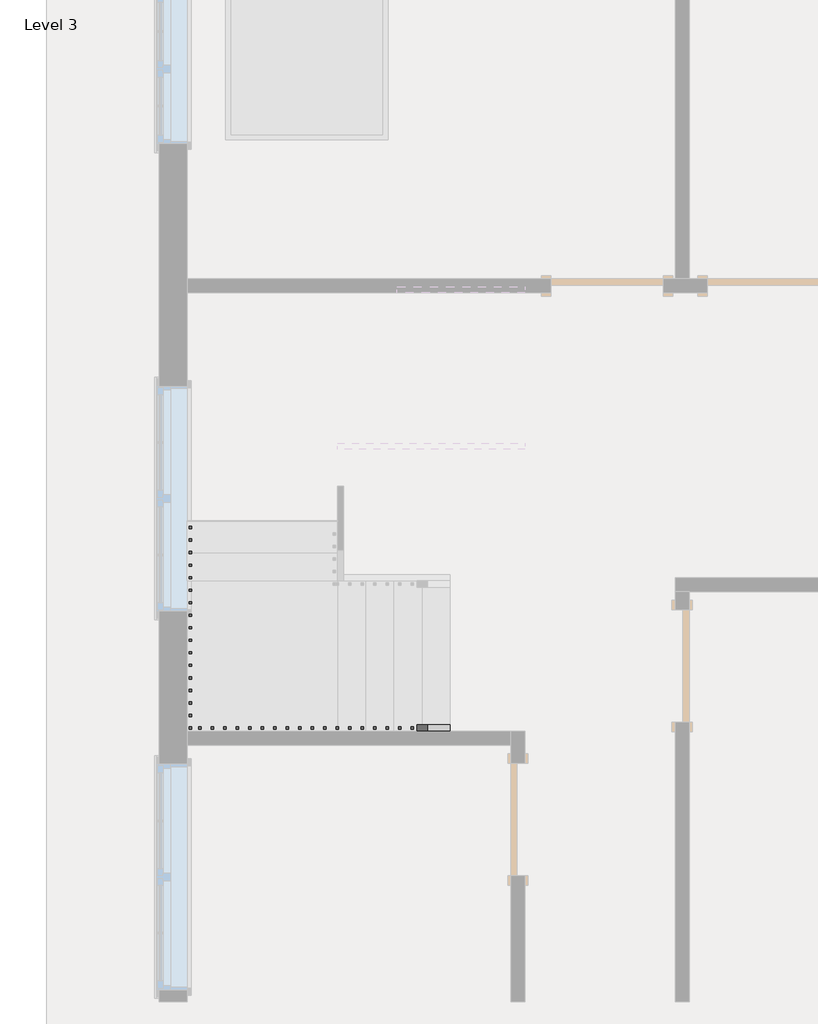
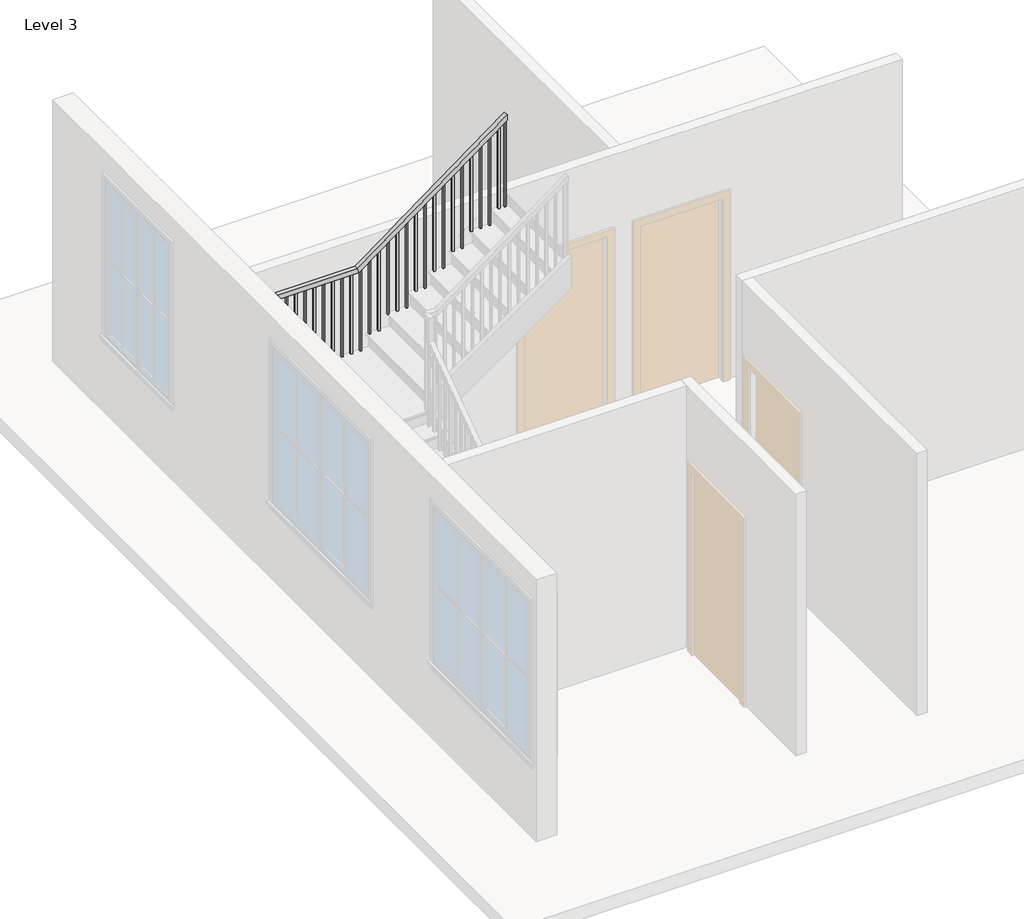
# One storey, part 2 of 3: 1 railing.
"""IFC4 building model written with IfcOpenShell, lengths in millimetres."""

from ifc_helpers import new_model, si_unit, frame, origin, place, context, project, spatial, polyline, outline, extrude, faceted_brep, element, save

model = new_model("IFC4")

# Units and contexts
model_context = context("Model", 3, world=origin())
ifc_project = project(units=[si_unit("LENGTHUNIT", "METRE", prefix="MILLI")], contexts=[model_context])

# Site, building, storey
site = spatial("IfcSite", under=ifc_project)
building = spatial("IfcBuilding", under=site)
storey = spatial("IfcBuildingStorey", under=building, Name="Level 3", Elevation=6248.4)

# Railing
placement = place(None, origin())
element("IfcRailing", 1, ObjectType="Handrail - Rectangular", at=placement, inside=storey, context=model_context, shape_type="SolidModel", body=[
    faceted_brep([(-2683.1105391, -2741.0373761, 7323.2210526), (-2683.1105391, -2741.0373761, 7261.1605986), (-2683.1105391, -2690.2373761, 7261.1605986), (-2683.1105391, -2690.2373761, 7323.2210526), (-3698.24463, -2741.0373761, 8035.5958533), (-3714.290777, -2741.0373761, 7984.7958533), (-3714.290777, -2690.2373761, 7984.7958533), (-3698.24463, -2690.2373761, 8035.5958533), (-4816.7105391, -2741.0373761, 8035.5958533), (-4816.7105391, -2741.0373761, 7984.7958533), (-4765.9105391, -2690.2373761, 7984.7958533), (-4765.9105391, -2690.2373761, 8035.5958533), (-4816.7105391, -1646.8618205, 8035.5958533), (-4816.7105391, -1630.5188912, 7984.7958533), (-4765.9105391, -1630.5188912, 7984.7958533), (-4765.9105391, -1646.8618205, 8035.5958533), (-4816.7105391, -308.3947094, 8996.2181818), (-4816.7105391, -292.0517801, 8945.4181818), (-4765.9105391, -292.0517801, 8945.4181818), (-4765.9105391, -308.3947094, 8996.2181818), (-4816.7105391, 814.9626239, 8996.2181818), (-4816.7105391, 814.9626239, 8945.4181818), (-4765.9105391, 764.1626239, 8945.4181818), (-4765.9105391, 764.1626239, 8996.2181818), (-3721.871578, 814.9626239, 8996.2181818), (-3705.1770744, 814.9626239, 8945.4181818), (-3705.1770744, 764.1626239, 8945.4181818), (-3721.871578, 764.1626239, 8996.2181818), (-2073.5105391, 814.9626239, 10210.8), (-2073.5105391, 764.1626239, 10210.8), (-2073.5105391, 764.1626239, 10147.6987868), (-2073.5105391, 814.9626239, 10147.6987868)], [[[0, 1, 2, 3]], [[1, 0, 4, 5]], [[2, 1, 5, 6]], [[3, 2, 6, 7]], [[0, 3, 7, 4]], [[5, 4, 8, 9]], [[6, 5, 9, 10]], [[7, 6, 10, 11]], [[4, 7, 11, 8]], [[9, 8, 12, 13]], [[10, 9, 13, 14]], [[11, 10, 14, 15]], [[8, 11, 15, 12]], [[13, 12, 16, 17]], [[14, 13, 17, 18]], [[15, 14, 18, 19]], [[12, 15, 19, 16]], [[17, 16, 20, 21]], [[18, 17, 21, 22]], [[19, 18, 22, 23]], [[16, 19, 23, 20]], [[21, 20, 24, 25]], [[22, 21, 25, 26]], [[23, 22, 26, 27]], [[20, 23, 27, 24]], [[28, 29, 30, 31]], [[25, 24, 28, 31]], [[26, 25, 31, 30]], [[27, 26, 30, 29]], [[24, 27, 29, 28]]]),
    extrude(outline(polyline([(10084.5329974, -2159.2355391), (9135.9789474, -2159.2355391), (9135.9789474, -2140.1855391), (10098.5698395, -2140.1855391), (10084.5329974, -2159.2355391)])), frame((0.0, 780.0376239, 0.0), z_axis=(0.0, 1.0, 0.0), x_axis=(0.0, 0.0, 1.0)), (0.0, 0.0, 1.0), 19.05),
    extrude(outline(polyline([(10009.6698395, -2260.8355391), (8975.5578947, -2260.8355391), (8975.5578947, -2241.7855391), (10023.7066816, -2241.7855391), (10009.6698395, -2260.8355391)])), frame((0.0, 780.0376239, 0.0), z_axis=(0.0, 1.0, 0.0), x_axis=(0.0, 0.0, 1.0)), (0.0, 0.0, 1.0), 19.05),
    extrude(outline(polyline([(9934.8066816, -2362.4355391), (8975.5578947, -2362.4355391), (8975.5578947, -2343.3855391), (9948.8435237, -2343.3855391), (9934.8066816, -2362.4355391)])), frame((0.0, 780.0376239, 0.0), z_axis=(0.0, 1.0, 0.0), x_axis=(0.0, 0.0, 1.0)), (0.0, 0.0, 1.0), 19.05),
    extrude(outline(polyline([(9859.9435237, -2464.0355391), (8975.5578947, -2464.0355391), (8975.5578947, -2444.9855391), (9873.9803658, -2444.9855391), (9859.9435237, -2464.0355391)])), frame((0.0, 780.0376239, 0.0), z_axis=(0.0, 1.0, 0.0), x_axis=(0.0, 0.0, 1.0)), (0.0, 0.0, 1.0), 19.05),
    extrude(outline(polyline([(9785.0803658, -2565.6355391), (8815.1368421, -2565.6355391), (8815.1368421, -2546.5855391), (9799.1172079, -2546.5855391), (9785.0803658, -2565.6355391)])), frame((0.0, 780.0376239, 0.0), z_axis=(0.0, 1.0, 0.0), x_axis=(0.0, 0.0, 1.0)), (0.0, 0.0, 1.0), 19.05),
    extrude(outline(polyline([(9710.2172079, -2667.2355391), (8815.1368421, -2667.2355391), (8815.1368421, -2648.1855391), (9724.25405, -2648.1855391), (9710.2172079, -2667.2355391)])), frame((0.0, 780.0376239, 0.0), z_axis=(0.0, 1.0, 0.0), x_axis=(0.0, 0.0, 1.0)), (0.0, 0.0, 1.0), 19.05),
    extrude(outline(polyline([(9635.35405, -2768.8355391), (8654.7157895, -2768.8355391), (8654.7157895, -2749.7855391), (9649.3908921, -2749.7855391), (9635.35405, -2768.8355391)])), frame((0.0, 780.0376239, 0.0), z_axis=(0.0, 1.0, 0.0), x_axis=(0.0, 0.0, 1.0)), (0.0, 0.0, 1.0), 19.05),
    extrude(outline(polyline([(9560.4908921, -2870.4355391), (8654.7157895, -2870.4355391), (8654.7157895, -2851.3855391), (9574.5277342, -2851.3855391), (9560.4908921, -2870.4355391)])), frame((0.0, 780.0376239, 0.0), z_axis=(0.0, 1.0, 0.0), x_axis=(0.0, 0.0, 1.0)), (0.0, 0.0, 1.0), 19.05),
    extrude(outline(polyline([(9485.6277342, -2972.0355391), (8494.2947368, -2972.0355391), (8494.2947368, -2952.9855391), (9499.6645763, -2952.9855391), (9485.6277342, -2972.0355391)])), frame((0.0, 780.0376239, 0.0), z_axis=(0.0, 1.0, 0.0), x_axis=(0.0, 0.0, 1.0)), (0.0, 0.0, 1.0), 19.05),
    extrude(outline(polyline([(9410.7645763, -3073.6355391), (8494.2947368, -3073.6355391), (8494.2947368, -3054.5855391), (9424.8014184, -3054.5855391), (9410.7645763, -3073.6355391)])), frame((0.0, 780.0376239, 0.0), z_axis=(0.0, 1.0, 0.0), x_axis=(0.0, 0.0, 1.0)), (0.0, 0.0, 1.0), 19.05),
    extrude(outline(polyline([(9335.9014184, -3175.2355391), (8333.8736842, -3175.2355391), (8333.8736842, -3156.1855391), (9349.9382605, -3156.1855391), (9335.9014184, -3175.2355391)])), frame((0.0, 780.0376239, 0.0), z_axis=(0.0, 1.0, 0.0), x_axis=(0.0, 0.0, 1.0)), (0.0, 0.0, 1.0), 19.05),
    extrude(outline(polyline([(9261.0382605, -3276.8355391), (8333.8736842, -3276.8355391), (8333.8736842, -3257.7855391), (9275.0751026, -3257.7855391), (9261.0382605, -3276.8355391)])), frame((0.0, 780.0376239, 0.0), z_axis=(0.0, 1.0, 0.0), x_axis=(0.0, 0.0, 1.0)), (0.0, 0.0, 1.0), 19.05),
    extrude(outline(polyline([(9186.1751026, -3378.4355391), (8333.8736842, -3378.4355391), (8333.8736842, -3359.3855391), (9200.2119447, -3359.3855391), (9186.1751026, -3378.4355391)])), frame((0.0, 780.0376239, 0.0), z_axis=(0.0, 1.0, 0.0), x_axis=(0.0, 0.0, 1.0)), (0.0, 0.0, 1.0), 19.05),
    extrude(outline(polyline([(9111.3119447, -3480.0355391), (8173.4526316, -3480.0355391), (8173.4526316, -3460.9855391), (9125.3487868, -3460.9855391), (9111.3119447, -3480.0355391)])), frame((0.0, 780.0376239, 0.0), z_axis=(0.0, 1.0, 0.0), x_axis=(0.0, 0.0, 1.0)), (0.0, 0.0, 1.0), 19.05),
    extrude(outline(polyline([(9036.4487868, -3581.6355391), (8173.4526316, -3581.6355391), (8173.4526316, -3562.5855391), (9050.4856289, -3562.5855391), (9036.4487868, -3581.6355391)])), frame((0.0, 780.0376239, 0.0), z_axis=(0.0, 1.0, 0.0), x_axis=(0.0, 0.0, 1.0)), (0.0, 0.0, 1.0), 19.05),
    extrude(outline(polyline([(8961.5856289, -3683.2355391), (8013.0315789, -3683.2355391), (8013.0315789, -3664.1855391), (8975.622471, -3664.1855391), (8961.5856289, -3683.2355391)])), frame((0.0, 780.0376239, 0.0), z_axis=(0.0, 1.0, 0.0), x_axis=(0.0, 0.0, 1.0)), (0.0, 0.0, 1.0), 19.05),
    extrude(outline(polyline([(-3784.8355391, 799.0876239), (-3765.7855391, 799.0876239), (-3765.7855391, 780.0376239), (-3784.8355391, 780.0376239), (-3784.8355391, 799.0876239)])), frame((0.0, 0.0, 8013.0315789), z_axis=(0.0, 0.0, 1.0), x_axis=(1.0, 0.0, 0.0)), (0.0, 0.0, 1.0), 932.3866029),
    extrude(outline(polyline([(-3886.4355391, 799.0876239), (-3867.3855391, 799.0876239), (-3867.3855391, 780.0376239), (-3886.4355391, 780.0376239), (-3886.4355391, 799.0876239)])), frame((0.0, 0.0, 8013.0315789), z_axis=(0.0, 0.0, 1.0), x_axis=(1.0, 0.0, 0.0)), (0.0, 0.0, 1.0), 932.3866029),
    extrude(outline(polyline([(-3988.0355391, 799.0876239), (-3968.9855391, 799.0876239), (-3968.9855391, 780.0376239), (-3988.0355391, 780.0376239), (-3988.0355391, 799.0876239)])), frame((0.0, 0.0, 8013.0315789), z_axis=(0.0, 0.0, 1.0), x_axis=(1.0, 0.0, 0.0)), (0.0, 0.0, 1.0), 932.3866029),
    extrude(outline(polyline([(-4089.6355391, 799.0876239), (-4070.5855391, 799.0876239), (-4070.5855391, 780.0376239), (-4089.6355391, 780.0376239), (-4089.6355391, 799.0876239)])), frame((0.0, 0.0, 8013.0315789), z_axis=(0.0, 0.0, 1.0), x_axis=(1.0, 0.0, 0.0)), (0.0, 0.0, 1.0), 932.3866029),
    extrude(outline(polyline([(-4191.2355391, 799.0876239), (-4172.1855391, 799.0876239), (-4172.1855391, 780.0376239), (-4191.2355391, 780.0376239), (-4191.2355391, 799.0876239)])), frame((0.0, 0.0, 8013.0315789), z_axis=(0.0, 0.0, 1.0), x_axis=(1.0, 0.0, 0.0)), (0.0, 0.0, 1.0), 932.3866029),
    extrude(outline(polyline([(-4292.8355391, 799.0876239), (-4273.7855391, 799.0876239), (-4273.7855391, 780.0376239), (-4292.8355391, 780.0376239), (-4292.8355391, 799.0876239)])), frame((0.0, 0.0, 8013.0315789), z_axis=(0.0, 0.0, 1.0), x_axis=(1.0, 0.0, 0.0)), (0.0, 0.0, 1.0), 932.3866029),
    extrude(outline(polyline([(-4394.4355391, 799.0876239), (-4375.3855391, 799.0876239), (-4375.3855391, 780.0376239), (-4394.4355391, 780.0376239), (-4394.4355391, 799.0876239)])), frame((0.0, 0.0, 8013.0315789), z_axis=(0.0, 0.0, 1.0), x_axis=(1.0, 0.0, 0.0)), (0.0, 0.0, 1.0), 932.3866029),
    extrude(outline(polyline([(-4496.0355391, 799.0876239), (-4476.9855391, 799.0876239), (-4476.9855391, 780.0376239), (-4496.0355391, 780.0376239), (-4496.0355391, 799.0876239)])), frame((0.0, 0.0, 8013.0315789), z_axis=(0.0, 0.0, 1.0), x_axis=(1.0, 0.0, 0.0)), (0.0, 0.0, 1.0), 932.3866029),
    extrude(outline(polyline([(-4597.6355391, 799.0876239), (-4578.5855391, 799.0876239), (-4578.5855391, 780.0376239), (-4597.6355391, 780.0376239), (-4597.6355391, 799.0876239)])), frame((0.0, 0.0, 8013.0315789), z_axis=(0.0, 0.0, 1.0), x_axis=(1.0, 0.0, 0.0)), (0.0, 0.0, 1.0), 932.3866029),
    extrude(outline(polyline([(-4699.2355391, 799.0876239), (-4680.1855391, 799.0876239), (-4680.1855391, 780.0376239), (-4699.2355391, 780.0376239), (-4699.2355391, 799.0876239)])), frame((0.0, 0.0, 8013.0315789), z_axis=(0.0, 0.0, 1.0), x_axis=(1.0, 0.0, 0.0)), (0.0, 0.0, 1.0), 932.3866029),
    extrude(outline(polyline([(-4800.8355391, 729.2376239), (-4800.8355391, 748.2876239), (-4781.7855391, 748.2876239), (-4781.7855391, 729.2376239), (-4800.8355391, 729.2376239)])), frame((0.0, 0.0, 8013.0315789), z_axis=(0.0, 0.0, 1.0), x_axis=(1.0, 0.0, 0.0)), (0.0, 0.0, 1.0), 932.3866029),
    extrude(outline(polyline([(-4800.8355391, 627.6376239), (-4800.8355391, 646.6876239), (-4781.7855391, 646.6876239), (-4781.7855391, 627.6376239), (-4800.8355391, 627.6376239)])), frame((0.0, 0.0, 8013.0315789), z_axis=(0.0, 0.0, 1.0), x_axis=(1.0, 0.0, 0.0)), (0.0, 0.0, 1.0), 932.3866029),
    extrude(outline(polyline([(-4800.8355391, 526.0376239), (-4800.8355391, 545.0876239), (-4781.7855391, 545.0876239), (-4781.7855391, 526.0376239), (-4800.8355391, 526.0376239)])), frame((0.0, 0.0, 8013.0315789), z_axis=(0.0, 0.0, 1.0), x_axis=(1.0, 0.0, 0.0)), (0.0, 0.0, 1.0), 932.3866029),
    extrude(outline(polyline([(-4800.8355391, 424.4376239), (-4800.8355391, 443.4876239), (-4781.7855391, 443.4876239), (-4781.7855391, 424.4376239), (-4800.8355391, 424.4376239)])), frame((0.0, 0.0, 8013.0315789), z_axis=(0.0, 0.0, 1.0), x_axis=(1.0, 0.0, 0.0)), (0.0, 0.0, 1.0), 932.3866029),
    extrude(outline(polyline([(-4800.8355391, 322.8376239), (-4800.8355391, 341.8876239), (-4781.7855391, 341.8876239), (-4781.7855391, 322.8376239), (-4800.8355391, 322.8376239)])), frame((0.0, 0.0, 8013.0315789), z_axis=(0.0, 0.0, 1.0), x_axis=(1.0, 0.0, 0.0)), (0.0, 0.0, 1.0), 932.3866029),
    extrude(outline(polyline([(-4800.8355391, 221.2376239), (-4800.8355391, 240.2876239), (-4781.7855391, 240.2876239), (-4781.7855391, 221.2376239), (-4800.8355391, 221.2376239)])), frame((0.0, 0.0, 8013.0315789), z_axis=(0.0, 0.0, 1.0), x_axis=(1.0, 0.0, 0.0)), (0.0, 0.0, 1.0), 932.3866029),
    extrude(outline(polyline([(-4800.8355391, 119.6376239), (-4800.8355391, 138.6876239), (-4781.7855391, 138.6876239), (-4781.7855391, 119.6376239), (-4800.8355391, 119.6376239)])), frame((0.0, 0.0, 8013.0315789), z_axis=(0.0, 0.0, 1.0), x_axis=(1.0, 0.0, 0.0)), (0.0, 0.0, 1.0), 932.3866029),
    extrude(outline(polyline([(-4800.8355391, 18.0376239), (-4800.8355391, 37.0876239), (-4781.7855391, 37.0876239), (-4781.7855391, 18.0376239), (-4800.8355391, 18.0376239)])), frame((0.0, 0.0, 8013.0315789), z_axis=(0.0, 0.0, 1.0), x_axis=(1.0, 0.0, 0.0)), (0.0, 0.0, 1.0), 932.3866029),
    extrude(outline(polyline([(-4800.8355391, -83.5623761), (-4800.8355391, -64.5123761), (-4781.7855391, -64.5123761), (-4781.7855391, -83.5623761), (-4800.8355391, -83.5623761)])), frame((0.0, 0.0, 8013.0315789), z_axis=(0.0, 0.0, 1.0), x_axis=(1.0, 0.0, 0.0)), (0.0, 0.0, 1.0), 932.3866029),
    extrude(outline(polyline([(-4800.8355391, -185.1623761), (-4800.8355391, -166.1123761), (-4781.7855391, -166.1123761), (-4781.7855391, -185.1623761), (-4800.8355391, -185.1623761)])), frame((0.0, 0.0, 8013.0315789), z_axis=(0.0, 0.0, 1.0), x_axis=(1.0, 0.0, 0.0)), (0.0, 0.0, 1.0), 932.3866029),
    extrude(outline(polyline([(-4800.8355391, -286.7623761), (-4800.8355391, -267.7123761), (-4781.7855391, -267.7123761), (-4781.7855391, -286.7623761), (-4800.8355391, -286.7623761)])), frame((0.0, 0.0, 8013.0315789), z_axis=(0.0, 0.0, 1.0), x_axis=(1.0, 0.0, 0.0)), (0.0, 0.0, 1.0), 932.3866029),
    extrude(outline(polyline([(-369.3123761, 8889.9679933), (-369.3123761, 8013.0315789), (-388.3623761, 8013.0315789), (-388.3623761, 8876.2957445), (-369.3123761, 8889.9679933)])), frame((-4800.8355391, 0.0, 0.0), z_axis=(1.0, 0.0, 0.0), x_axis=(0.0, 1.0, 0.0)), (0.0, 0.0, 1.0), 19.05),
    extrude(outline(polyline([(-470.9123761, 8817.049333), (-470.9123761, 7852.6105263), (-489.9623761, 7852.6105263), (-489.9623761, 8803.3770842), (-470.9123761, 8817.049333)])), frame((-4800.8355391, 0.0, 0.0), z_axis=(1.0, 0.0, 0.0), x_axis=(0.0, 1.0, 0.0)), (0.0, 0.0, 1.0), 19.05),
    extrude(outline(polyline([(-572.5123761, 8744.1306727), (-572.5123761, 7852.6105263), (-591.5623761, 7852.6105263), (-591.5623761, 8730.4584239), (-572.5123761, 8744.1306727)])), frame((-4800.8355391, 0.0, 0.0), z_axis=(1.0, 0.0, 0.0), x_axis=(0.0, 1.0, 0.0)), (0.0, 0.0, 1.0), 19.05),
    extrude(outline(polyline([(-674.1123761, 8671.2120124), (-674.1123761, 7692.1894737), (-693.1623761, 7692.1894737), (-693.1623761, 8657.5397636), (-674.1123761, 8671.2120124)])), frame((-4800.8355391, 0.0, 0.0), z_axis=(1.0, 0.0, 0.0), x_axis=(0.0, 1.0, 0.0)), (0.0, 0.0, 1.0), 19.05),
    extrude(outline(polyline([(-775.7123761, 8598.2933521), (-775.7123761, 7692.1894737), (-794.7623761, 7692.1894737), (-794.7623761, 8584.6211033), (-775.7123761, 8598.2933521)])), frame((-4800.8355391, 0.0, 0.0), z_axis=(1.0, 0.0, 0.0), x_axis=(0.0, 1.0, 0.0)), (0.0, 0.0, 1.0), 19.05),
    extrude(outline(polyline([(-877.3123761, 8525.3746919), (-877.3123761, 7531.7684211), (-896.3623761, 7531.7684211), (-896.3623761, 8511.702443), (-877.3123761, 8525.3746919)])), frame((-4800.8355391, 0.0, 0.0), z_axis=(1.0, 0.0, 0.0), x_axis=(0.0, 1.0, 0.0)), (0.0, 0.0, 1.0), 19.05),
    extrude(outline(polyline([(-978.9123761, 8452.4560316), (-978.9123761, 7531.7684211), (-997.9623761, 7531.7684211), (-997.9623761, 8438.7837828), (-978.9123761, 8452.4560316)])), frame((-4800.8355391, 0.0, 0.0), z_axis=(1.0, 0.0, 0.0), x_axis=(0.0, 1.0, 0.0)), (0.0, 0.0, 1.0), 19.05),
    extrude(outline(polyline([(-1080.5123761, 8379.5373713), (-1080.5123761, 7371.3473684), (-1099.5623761, 7371.3473684), (-1099.5623761, 8365.8651225), (-1080.5123761, 8379.5373713)])), frame((-4800.8355391, 0.0, 0.0), z_axis=(1.0, 0.0, 0.0), x_axis=(0.0, 1.0, 0.0)), (0.0, 0.0, 1.0), 19.05),
    extrude(outline(polyline([(-1182.1123761, 8306.618711), (-1182.1123761, 7371.3473684), (-1201.1623761, 7371.3473684), (-1201.1623761, 8292.9464622), (-1182.1123761, 8306.618711)])), frame((-4800.8355391, 0.0, 0.0), z_axis=(1.0, 0.0, 0.0), x_axis=(0.0, 1.0, 0.0)), (0.0, 0.0, 1.0), 19.05),
    extrude(outline(polyline([(-1283.7123761, 8233.7000507), (-1283.7123761, 7371.3473684), (-1302.7623761, 7371.3473684), (-1302.7623761, 8220.0278019), (-1283.7123761, 8233.7000507)])), frame((-4800.8355391, 0.0, 0.0), z_axis=(1.0, 0.0, 0.0), x_axis=(0.0, 1.0, 0.0)), (0.0, 0.0, 1.0), 19.05),
    extrude(outline(polyline([(-1385.3123761, 8160.7813904), (-1385.3123761, 7210.9263158), (-1404.3623761, 7210.9263158), (-1404.3623761, 8147.1091416), (-1385.3123761, 8160.7813904)])), frame((-4800.8355391, 0.0, 0.0), z_axis=(1.0, 0.0, 0.0), x_axis=(0.0, 1.0, 0.0)), (0.0, 0.0, 1.0), 19.05),
    extrude(outline(polyline([(-1486.9123761, 8087.8627301), (-1486.9123761, 7210.9263158), (-1505.9623761, 7210.9263158), (-1505.9623761, 8074.1904813), (-1486.9123761, 8087.8627301)])), frame((-4800.8355391, 0.0, 0.0), z_axis=(1.0, 0.0, 0.0), x_axis=(0.0, 1.0, 0.0)), (0.0, 0.0, 1.0), 19.05),
    extrude(outline(polyline([(-1588.5123761, 8014.9440698), (-1588.5123761, 7050.5052632), (-1607.5623761, 7050.5052632), (-1607.5623761, 8001.271821), (-1588.5123761, 8014.9440698)])), frame((-4800.8355391, 0.0, 0.0), z_axis=(1.0, 0.0, 0.0), x_axis=(0.0, 1.0, 0.0)), (0.0, 0.0, 1.0), 19.05),
    extrude(outline(polyline([(-4800.8355391, -1709.1623761), (-4800.8355391, -1690.1123761), (-4781.7855391, -1690.1123761), (-4781.7855391, -1709.1623761), (-4800.8355391, -1709.1623761)])), frame((0.0, 0.0, 7050.5052632), z_axis=(0.0, 0.0, 1.0), x_axis=(1.0, 0.0, 0.0)), (0.0, 0.0, 1.0), 934.2905901),
    extrude(outline(polyline([(-4800.8355391, -1810.7623761), (-4800.8355391, -1791.7123761), (-4781.7855391, -1791.7123761), (-4781.7855391, -1810.7623761), (-4800.8355391, -1810.7623761)])), frame((0.0, 0.0, 7050.5052632), z_axis=(0.0, 0.0, 1.0), x_axis=(1.0, 0.0, 0.0)), (0.0, 0.0, 1.0), 934.2905901),
    extrude(outline(polyline([(-4800.8355391, -1912.3623761), (-4800.8355391, -1893.3123761), (-4781.7855391, -1893.3123761), (-4781.7855391, -1912.3623761), (-4800.8355391, -1912.3623761)])), frame((0.0, 0.0, 7050.5052632), z_axis=(0.0, 0.0, 1.0), x_axis=(1.0, 0.0, 0.0)), (0.0, 0.0, 1.0), 934.2905901),
    extrude(outline(polyline([(-4800.8355391, -2013.9623761), (-4800.8355391, -1994.9123761), (-4781.7855391, -1994.9123761), (-4781.7855391, -2013.9623761), (-4800.8355391, -2013.9623761)])), frame((0.0, 0.0, 7050.5052632), z_axis=(0.0, 0.0, 1.0), x_axis=(1.0, 0.0, 0.0)), (0.0, 0.0, 1.0), 934.2905901),
    extrude(outline(polyline([(-4800.8355391, -2115.5623761), (-4800.8355391, -2096.5123761), (-4781.7855391, -2096.5123761), (-4781.7855391, -2115.5623761), (-4800.8355391, -2115.5623761)])), frame((0.0, 0.0, 7050.5052632), z_axis=(0.0, 0.0, 1.0), x_axis=(1.0, 0.0, 0.0)), (0.0, 0.0, 1.0), 934.2905901),
    extrude(outline(polyline([(-4800.8355391, -2217.1623761), (-4800.8355391, -2198.1123761), (-4781.7855391, -2198.1123761), (-4781.7855391, -2217.1623761), (-4800.8355391, -2217.1623761)])), frame((0.0, 0.0, 7050.5052632), z_axis=(0.0, 0.0, 1.0), x_axis=(1.0, 0.0, 0.0)), (0.0, 0.0, 1.0), 934.2905901),
    extrude(outline(polyline([(-4800.8355391, -2318.7623761), (-4800.8355391, -2299.7123761), (-4781.7855391, -2299.7123761), (-4781.7855391, -2318.7623761), (-4800.8355391, -2318.7623761)])), frame((0.0, 0.0, 7050.5052632), z_axis=(0.0, 0.0, 1.0), x_axis=(1.0, 0.0, 0.0)), (0.0, 0.0, 1.0), 934.2905901),
    extrude(outline(polyline([(-4800.8355391, -2420.3623761), (-4800.8355391, -2401.3123761), (-4781.7855391, -2401.3123761), (-4781.7855391, -2420.3623761), (-4800.8355391, -2420.3623761)])), frame((0.0, 0.0, 7050.5052632), z_axis=(0.0, 0.0, 1.0), x_axis=(1.0, 0.0, 0.0)), (0.0, 0.0, 1.0), 934.2905901),
    extrude(outline(polyline([(-4800.8355391, -2521.9623761), (-4800.8355391, -2502.9123761), (-4781.7855391, -2502.9123761), (-4781.7855391, -2521.9623761), (-4800.8355391, -2521.9623761)])), frame((0.0, 0.0, 7050.5052632), z_axis=(0.0, 0.0, 1.0), x_axis=(1.0, 0.0, 0.0)), (0.0, 0.0, 1.0), 934.2905901),
    extrude(outline(polyline([(-4800.8355391, -2623.5623761), (-4800.8355391, -2604.5123761), (-4781.7855391, -2604.5123761), (-4781.7855391, -2623.5623761), (-4800.8355391, -2623.5623761)])), frame((0.0, 0.0, 7050.5052632), z_axis=(0.0, 0.0, 1.0), x_axis=(1.0, 0.0, 0.0)), (0.0, 0.0, 1.0), 934.2905901),
    extrude(outline(polyline([(-4705.5855391, -2725.1623761), (-4724.6355391, -2725.1623761), (-4724.6355391, -2706.1123761), (-4705.5855391, -2706.1123761), (-4705.5855391, -2725.1623761)])), frame((0.0, 0.0, 7050.5052632), z_axis=(0.0, 0.0, 1.0), x_axis=(1.0, 0.0, 0.0)), (0.0, 0.0, 1.0), 934.2905901),
    extrude(outline(polyline([(-4603.9855391, -2725.1623761), (-4623.0355391, -2725.1623761), (-4623.0355391, -2706.1123761), (-4603.9855391, -2706.1123761), (-4603.9855391, -2725.1623761)])), frame((0.0, 0.0, 7050.5052632), z_axis=(0.0, 0.0, 1.0), x_axis=(1.0, 0.0, 0.0)), (0.0, 0.0, 1.0), 934.2905901),
    extrude(outline(polyline([(-4502.3855391, -2725.1623761), (-4521.4355391, -2725.1623761), (-4521.4355391, -2706.1123761), (-4502.3855391, -2706.1123761), (-4502.3855391, -2725.1623761)])), frame((0.0, 0.0, 7050.5052632), z_axis=(0.0, 0.0, 1.0), x_axis=(1.0, 0.0, 0.0)), (0.0, 0.0, 1.0), 934.2905901),
    extrude(outline(polyline([(-4400.7855391, -2725.1623761), (-4419.8355391, -2725.1623761), (-4419.8355391, -2706.1123761), (-4400.7855391, -2706.1123761), (-4400.7855391, -2725.1623761)])), frame((0.0, 0.0, 7050.5052632), z_axis=(0.0, 0.0, 1.0), x_axis=(1.0, 0.0, 0.0)), (0.0, 0.0, 1.0), 934.2905901),
    extrude(outline(polyline([(-4299.1855391, -2725.1623761), (-4318.2355391, -2725.1623761), (-4318.2355391, -2706.1123761), (-4299.1855391, -2706.1123761), (-4299.1855391, -2725.1623761)])), frame((0.0, 0.0, 7050.5052632), z_axis=(0.0, 0.0, 1.0), x_axis=(1.0, 0.0, 0.0)), (0.0, 0.0, 1.0), 934.2905901),
    extrude(outline(polyline([(-4197.5855391, -2725.1623761), (-4216.6355391, -2725.1623761), (-4216.6355391, -2706.1123761), (-4197.5855391, -2706.1123761), (-4197.5855391, -2725.1623761)])), frame((0.0, 0.0, 7050.5052632), z_axis=(0.0, 0.0, 1.0), x_axis=(1.0, 0.0, 0.0)), (0.0, 0.0, 1.0), 934.2905901),
    extrude(outline(polyline([(-4095.9855391, -2725.1623761), (-4115.0355391, -2725.1623761), (-4115.0355391, -2706.1123761), (-4095.9855391, -2706.1123761), (-4095.9855391, -2725.1623761)])), frame((0.0, 0.0, 7050.5052632), z_axis=(0.0, 0.0, 1.0), x_axis=(1.0, 0.0, 0.0)), (0.0, 0.0, 1.0), 934.2905901),
    extrude(outline(polyline([(-3994.3855391, -2725.1623761), (-4013.4355391, -2725.1623761), (-4013.4355391, -2706.1123761), (-3994.3855391, -2706.1123761), (-3994.3855391, -2725.1623761)])), frame((0.0, 0.0, 7050.5052632), z_axis=(0.0, 0.0, 1.0), x_axis=(1.0, 0.0, 0.0)), (0.0, 0.0, 1.0), 934.2905901),
    extrude(outline(polyline([(-3892.7855391, -2725.1623761), (-3911.8355391, -2725.1623761), (-3911.8355391, -2706.1123761), (-3892.7855391, -2706.1123761), (-3892.7855391, -2725.1623761)])), frame((0.0, 0.0, 7050.5052632), z_axis=(0.0, 0.0, 1.0), x_axis=(1.0, 0.0, 0.0)), (0.0, 0.0, 1.0), 934.2905901),
    extrude(outline(polyline([(-3791.1855391, -2725.1623761), (-3810.2355391, -2725.1623761), (-3810.2355391, -2706.1123761), (-3791.1855391, -2706.1123761), (-3791.1855391, -2725.1623761)])), frame((0.0, 0.0, 7050.5052632), z_axis=(0.0, 0.0, 1.0), x_axis=(1.0, 0.0, 0.0)), (0.0, 0.0, 1.0), 934.2905901),
    extrude(outline(polyline([(-3689.5855391, -2725.1623761), (-3708.6355391, -2725.1623761), (-3708.6355391, -2706.1123761), (-3689.5855391, -2706.1123761), (-3689.5855391, -2725.1623761)])), frame((0.0, 0.0, 7050.5052632), z_axis=(0.0, 0.0, 1.0), x_axis=(1.0, 0.0, 0.0)), (0.0, 0.0, 1.0), 934.2905901),
    extrude(outline(polyline([(7909.5290196, -3607.0355391), (7050.5052632, -3607.0355391), (7050.5052632, -3587.9855391), (7896.1605986, -3587.9855391), (7909.5290196, -3607.0355391)])), frame((0.0, -2725.1623761, 0.0), z_axis=(0.0, 1.0, 0.0), x_axis=(0.0, 0.0, 1.0)), (0.0, 0.0, 1.0), 19.05),
    extrude(outline(polyline([(7838.230774, -3505.4355391), (6890.0842105, -3505.4355391), (6890.0842105, -3486.3855391), (7824.862353, -3486.3855391), (7838.230774, -3505.4355391)])), frame((0.0, -2725.1623761, 0.0), z_axis=(0.0, 1.0, 0.0), x_axis=(0.0, 0.0, 1.0)), (0.0, 0.0, 1.0), 19.05),
    extrude(outline(polyline([(7766.9325284, -3403.8355391), (6890.0842105, -3403.8355391), (6890.0842105, -3384.7855391), (7753.5641074, -3384.7855391), (7766.9325284, -3403.8355391)])), frame((0.0, -2725.1623761, 0.0), z_axis=(0.0, 1.0, 0.0), x_axis=(0.0, 0.0, 1.0)), (0.0, 0.0, 1.0), 19.05),
    extrude(outline(polyline([(7695.6342828, -3302.2355391), (6729.6631579, -3302.2355391), (6729.6631579, -3283.1855391), (7682.2658617, -3283.1855391), (7695.6342828, -3302.2355391)])), frame((0.0, -2725.1623761, 0.0), z_axis=(0.0, 1.0, 0.0), x_axis=(0.0, 0.0, 1.0)), (0.0, 0.0, 1.0), 19.05),
    extrude(outline(polyline([(7624.3360372, -3200.6355391), (6729.6631579, -3200.6355391), (6729.6631579, -3181.5855391), (7610.9676161, -3181.5855391), (7624.3360372, -3200.6355391)])), frame((0.0, -2725.1623761, 0.0), z_axis=(0.0, 1.0, 0.0), x_axis=(0.0, 0.0, 1.0)), (0.0, 0.0, 1.0), 19.05),
    extrude(outline(polyline([(7553.0377916, -3099.0355391), (6569.2421053, -3099.0355391), (6569.2421053, -3079.9855391), (7539.6693705, -3079.9855391), (7553.0377916, -3099.0355391)])), frame((0.0, -2725.1623761, 0.0), z_axis=(0.0, 1.0, 0.0), x_axis=(0.0, 0.0, 1.0)), (0.0, 0.0, 1.0), 19.05),
    extrude(outline(polyline([(7481.7395459, -2997.4355391), (6569.2421053, -2997.4355391), (6569.2421053, -2978.3855391), (7468.3711249, -2978.3855391), (7481.7395459, -2997.4355391)])), frame((0.0, -2725.1623761, 0.0), z_axis=(0.0, 1.0, 0.0), x_axis=(0.0, 0.0, 1.0)), (0.0, 0.0, 1.0), 19.05),
    extrude(outline(polyline([(7410.4413003, -2895.8355391), (6408.8210526, -2895.8355391), (6408.8210526, -2876.7855391), (7397.0728793, -2876.7855391), (7410.4413003, -2895.8355391)])), frame((0.0, -2725.1623761, 0.0), z_axis=(0.0, 1.0, 0.0), x_axis=(0.0, 0.0, 1.0)), (0.0, 0.0, 1.0), 19.05),
    extrude(outline(polyline([(7339.1430547, -2794.2355391), (6408.8210526, -2794.2355391), (6408.8210526, -2775.1855391), (7325.7746337, -2775.1855391), (7339.1430547, -2794.2355391)])), frame((0.0, -2725.1623761, 0.0), z_axis=(0.0, 1.0, 0.0), x_axis=(0.0, 0.0, 1.0)), (0.0, 0.0, 1.0), 19.05),
    extrude(outline(polyline([(-4800.8355391, 780.0376239), (-4800.8355391, 799.0876239), (-4781.7855391, 799.0876239), (-4781.7855391, 780.0376239), (-4800.8355391, 780.0376239)])), frame((0.0, 0.0, 8013.0315789), z_axis=(0.0, 0.0, 1.0), x_axis=(1.0, 0.0, 0.0)), (0.0, 0.0, 1.0), 932.3866029),
    extrude(outline(polyline([(-4781.7855391, -2725.1623761), (-4800.8355391, -2725.1623761), (-4800.8355391, -2706.1123761), (-4781.7855391, -2706.1123761), (-4781.7855391, -2725.1623761)])), frame((0.0, 0.0, 7050.5052632), z_axis=(0.0, 0.0, 1.0), x_axis=(1.0, 0.0, 0.0)), (0.0, 0.0, 1.0), 934.2905901),
    extrude(outline(polyline([(10133.6619447, -2092.5605391), (9135.9789474, -2092.5605391), (9135.9789474, -2073.5105391), (10147.6987868, -2073.5105391), (10133.6619447, -2092.5605391)])), frame((0.0, 780.0376239, 0.0), z_axis=(0.0, 1.0, 0.0), x_axis=(0.0, 0.0, 1.0)), (0.0, 0.0, 1.0), 19.05),
    extrude(outline(polyline([(7274.5290196, -2702.1605391), (6408.8210526, -2702.1605391), (6408.8210526, -2683.1105391), (7261.1605986, -2683.1105391), (7274.5290196, -2702.1605391)])), frame((0.0, -2725.1623761, 0.0), z_axis=(0.0, 1.0, 0.0), x_axis=(0.0, 0.0, 1.0)), (0.0, 0.0, 1.0), 19.05),
])

save(model, "model.ifc")

# Revit data of these elements
# Type "Handrail - Rectangular"
#   Assembly Code = "C2010400"
#   built-in parameter 1008612 = 0.0416667 (stored number, unit not read)
#   built-in parameter 1008611 = 0.0416667 (stored number, unit not read)
#   built-in parameter 1008609 = 0.333333 (stored number, unit not read)
#   built-in parameter 1008604 = 0.166667 (stored number, unit not read)
#   built-in parameter 1008603 = 0.166667 (stored number, unit not read)
#   Railing Height = 3' - 0"
#   built-in parameter 1008630 = 2
#   built-in parameter 1008610 = 2
#   built-in parameter 1008618 = Baluster - Square : 3/4"
# Element 1 (IfcRailing, "Handrail - Rectangular")
#   Phase Created = New Construction
